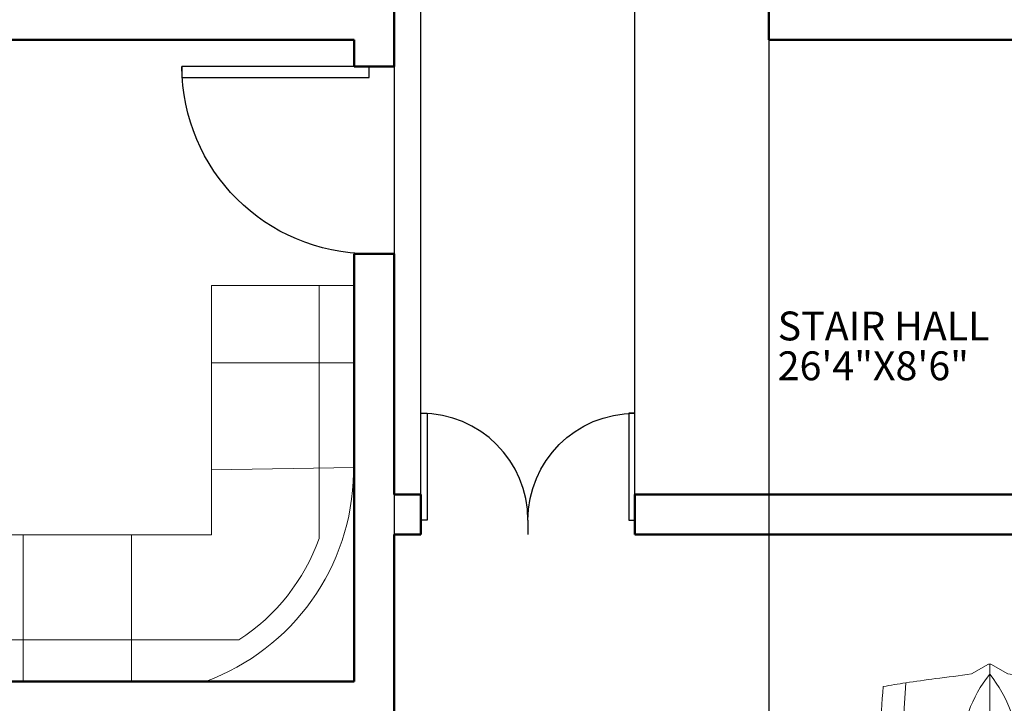
# Model space of a CAD drawing. Units: inches. Extents: x 5375 to 6084, y 16106 to 17259.
# Tile 8 of 32: x 5624 to 5844, y 16365 to 16518. Entities that reach past the tile are written whole.
import ezdxf

# ---------------------------------------------------------------- set-up
doc = ezdxf.new("R2010")
doc.units = ezdxf.units.IN
for name, color, linetype, lineweight in [('A-ANNO-DIMS', 2, 'Continuous', 18), ('A-AREA-IDEN', 5, 'Continuous', 18), ('C-PKNG-VEHI', 7, 'Continuous', 13), ('DOOR', 4, 'Continuous', 25), ('FURNITURE', 3, 'Continuous', 18), ('WALL', 6, 'Continuous', 50)]:
    doc.layers.add(name, color=color, linetype=linetype, lineweight=lineweight)
doc.styles.get("Standard").update_dxf_attribs({"font": 'arial.ttf'})
doc.dimstyles.get("Standard").update_dxf_attribs({"dimtxt": 0.18, "dimasz": 0.18, "dimexe": 0.18, "dimexo": 0.0625, "dimgap": 0.09, "dimtad": 0, "dimtih": 1, "dimtoh": 1, "dimdec": 4, "dimzin": 0, "dimdsep": 46, "dimtxsty": 'Standard', "dimcen": 0.09, "dimadec": 0, "dimazin": 0, "dimtfac": 1, "dimtdec": 4, "dimtofl": 0, "dimtmove": 0, "dimatfit": 3, "dimfxl": 1, "dimtolj": 1, "dimtzin": 0, "dimarcsym": 0})

# ---------------------------------------------------------------- blocks, each defined once
blk = doc.blocks.new('*U2')
for p, q in [((0, 0), (0, -100)), ((750, 0), (750, -100))]:
    blk.add_line(p, q)
blk.add_lwpolyline([(0, 0), (0, 750), (43.75, 750), (43.75, 0)], close=True)
blk.add_arc((0, 0), 750, 0, 90)
blk = doc.blocks.new('*U9')
for p, q in [((21.1, 37.41), (21.1, 36.83)), ((46.55, 38.89), (22.35, 38.89)), ((47.8, 37.39), (47.8, 37.41)), ((135.45, 37.07), (135.45, 37.41)), ((136.7, 38.89), (160.9, 38.89)), ((162.15, 37.41), (162.15, 36.77)), ((87.99, 31.87), (74.76, 35.92)), ((134.31, 35.6), (119.29, 31.78)), ((186.47, -33.5), (186.47, 33.5)), ((70.03, 31.54), (86.41, 29.35)), ((188.4, -32.76), (188.4, 32.76)), ((138.42, 29.35), (157.25, 29.35)), ((186.47, 29.35), (167.01, 29.35)), ((164.52, 26.39), (164.52, -26.39)), ((32.27, 11.63), (36.13, 17.17)), ((36.13, 17.17), (50.94, 17.17)), ((32.12, 9.51), (32.12, 11.15)), ((58.92, -10.77), (58.92, 10.77)), ((66.55, -10.53), (66.55, 10.53)), ((186.47, -10.53), (186.47, 10.53)), ((29.77, 9.51), (51.68, 9.51)), ((82.74, 8.5), (82.74, -8.5)), ((3.27, 6.13), (0.1, 0.41)), ((0, 0), (51.68, 0)), ((0.1, -0.41), (3.27, -6.13)), ((29.77, -9.51), (51.68, -9.51)), ((32.12, -9.51), (32.12, -11.15)), ((32.27, -11.63), (36.13, -17.17)), ((36.13, -17.17), (50.94, -17.17)), ((86.41, -29.35), (70.03, -31.54)), ((157.25, -29.35), (138.42, -29.35)), ((167.01, -29.35), (186.47, -29.35)), ((87.99, -31.87), (74.76, -35.92)), ((134.31, -35.6), (119.29, -31.78)), ((21.1, -37.41), (21.1, -36.83)), ((46.55, -38.89), (22.35, -38.89)), ((47.8, -37.39), (47.8, -37.41)), ((135.45, -37.07), (135.45, -37.41)), ((136.7, -38.89), (160.9, -38.89)), ((162.15, -37.41), (162.15, -36.77))]:
    blk.add_line(p, q)
for centre, major_axis, ratio, start_param, end_param in [((41.19, -490.86), (0, 528.23), 0.842304, 0.00281, 0.075598), ((22.35, 37.41), (0, -1.48), 0.842304, 3.141593, 4.712389), ((64.48, -10555.62), (0, 10593.03), 0.842304, -0.013397, 0.002797), ((46.55, 37.41), (0, 1.48), 0.842304, -1.570796, 0), ((136.7, 37.41), (0, -1.48), 0.842304, 3.141593, 4.712389), ((160.9, 37.41), (0, 1.48), 0.842304, -1.570796, 0), ((180.63, 35.84), (0, 2.22), 0.842304, -0.013017, 1.249894), ((64.48, -10556.36), (0, 10595.31), 0.842304, -0.013397, -0.013017), ((183.98, 32.76), (0, -5.25), 0.842304, 1.570796, 3.128196), ((266.03, -27.52), (0, 313.31), 0.842304, 1.367076, 1.39176), ((64.48, -10555.62), (0, -10591.55), 0.842304, 3.133765, 3.140441), ((183.98, 33.5), (0, -2.96), 0.842304, 1.570796, 3.128196), ((135.29, 5.39), (0, 81.77), 0.842304, 1.245306, 1.50788), ((95.79, -3666.35), (0, -3698.24), 0.842304, 3.134049, 3.144098), ((259.18, -27.52), (0, -305.3), 0.842304, 4.528606, 4.561838), ((37.47, -593.96), (0, -623.33), 0.842304, 3.096046, 3.200911), ((134.4, 5.39), (0, -89.78), 0.842304, 4.449482, 4.652344), ((149.6, 2.8), (0, -79.58), 0.842304, 4.372215, 4.640744), ((17.08, 0), (0, 147.02), 0.842304, 4.511394, 4.913384), ((35.91, 0), (0, 147.02), 0.842304, 4.511394, 4.913384), ((167.01, 26.39), (0, 2.96), 0.842304, 0, 1.570796), ((-204.49, 52.4), (0, -250.96), 0.842304, 1.385369, 1.434372), ((13.04, 17.01), (0, 27.42), 0.842304, 4.435146, 4.718221), ((14.2, 17.01), (0, 27.42), 0.842304, 4.435146, 4.718221), ((50.79, 13.34), (6.34, -0.36), 0.603834, -1.395552, 1.581315), ((32.75, 11.15), (0, 0.74), 0.842304, 0.879714, 1.570796), ((29.77, -46.66), (0, 56.17), 0.842304, 0, 0.590319), ((0.62, 0), (0, -0.74), 0.842304, 4.131459, 5.293319), ((29.77, 46.66), (0, 56.17), 0.842304, 2.551274, 3.141593), ((-204.49, -52.4), (0, 250.96), 0.842304, -1.434372, -1.385369), ((13.04, -17.01), (0, -27.42), 0.842304, 1.564964, 1.848039), ((14.2, -17.01), (0, -27.42), 0.842304, 1.564964, 1.848039), ((149.6, -2.8), (0, -79.58), 0.842304, -1.499151, -1.230623), ((32.75, -11.15), (0, -0.74), 0.842304, 4.712389, 5.403472), ((134.4, -5.39), (0, -89.78), 0.842304, -1.510751, -1.307889), ((135.29, -5.39), (0, -81.77), 0.842304, -1.50788, -1.245306), ((259.18, 27.52), (0, 305.3), 0.842304, 1.721348, 1.754579), ((167.01, -26.39), (0, -2.96), 0.842304, 4.712389, 6.283185), ((266.03, 27.52), (0, 313.31), 0.842304, 1.749832, 1.774517), ((37.47, 593.96), (0, -623.33), 0.842304, -0.059319, 0.045547), ((95.79, 3666.35), (0, -3698.24), 0.842304, -0.002505, 0.007544), ((183.98, -32.76), (0, -5.25), 0.842304, 0.013397, 1.570796), ((41.19, 490.86), (0, -528.23), 0.842304, -0.075598, -0.00281), ((64.48, 10555.62), (0, 10593.03), 0.842304, 3.138796, 3.15499), ((64.48, 10555.62), (0, -10591.55), 0.842304, 0.001152, 0.007828), ((183.98, -33.5), (0, 2.96), 0.842304, 3.15499, 4.712389), ((22.35, -37.41), (0, 1.48), 0.842304, 1.570796, 3.141593), ((46.55, -37.41), (0, -1.48), 0.842304, 0, 1.570796), ((136.7, -37.41), (0, -1.48), 0.842304, -1.570796, 0), ((160.9, -37.41), (0, 1.48), 0.842304, 3.141593, 4.712389), ((180.63, -35.84), (0, -2.22), 0.842304, -1.249894, 0.013017), ((64.48, 10556.36), (0, 10595.31), 0.842304, 3.15461, 3.15499)]:
    blk.add_ellipse(centre, major_axis=major_axis, ratio=ratio, start_param=start_param, end_param=end_param)
at = {"extrusion": (0, 0, -1)}
blk.add_ellipse((50.79, -13.34), major_axis=(6.34, 0.36), ratio=0.603834, start_param=-1.395552, end_param=1.581315, dxfattribs=at)
blk = doc.blocks.new('*D38')
at = {"layer": 'A-ANNO-DIMS', "color": 0, "lineweight": -2, "transparency": 16777216}
for p, q in [((5791.62, 16513.52), (5791.62, 16106.48)), ((5707.62, 16507.52), (5707.62, 16106.48)), ((5707.8, 16106.66), (5749.4, 16106.66)), ((5791.44, 16106.66), (5749.84, 16106.66))]:
    blk.add_line(p, q, dxfattribs=at)
at = {"layer": 'A-ANNO-DIMS', "color": 0, "transparency": 16777216}
for points in [[(5707.8, 16106.69), (5707.8, 16106.63), (5707.62, 16106.66)], [(5791.44, 16106.69), (5791.44, 16106.63), (5791.62, 16106.66)]]:
    blk.add_solid(points, dxfattribs=at)
at = {"layer": 'Defpoints', "color": 0, "transparency": 16777216}
for p in [(5791.62, 16513.58), (5707.62, 16507.58), (5791.62, 16106.66)]:
    blk.add_point(p, dxfattribs=at)
at = {"layer": 'A-ANNO-DIMS', "color": 0, "transparency": 16777216, "insert": (5749.62, 16106.66), "char_height": 0.18, "attachment_point": 5}
blk.add_mtext('\\A1;84', dxfattribs=at)
blk = doc.blocks.new('*D39')
at = {"layer": 'A-ANNO-DIMS', "color": 0, "lineweight": -2, "transparency": 16777216}
for p, q in [((5713.62, 16402.64), (5713.62, 17259.16)), ((5713.8, 17258.98), (5737.4, 17258.98)), ((5761.44, 17258.98), (5737.84, 17258.98)), ((5761.62, 16402.64), (5761.62, 17259.16))]:
    blk.add_line(p, q, dxfattribs=at)
at = {"layer": 'A-ANNO-DIMS', "color": 0, "transparency": 16777216}
for points in [[(5713.8, 17259.01), (5713.8, 17258.95), (5713.62, 17258.98)], [(5761.44, 17259.01), (5761.44, 17258.95), (5761.62, 17258.98)]]:
    blk.add_solid(points, dxfattribs=at)
at = {"layer": 'Defpoints', "color": 0, "transparency": 16777216}
for p in [(5761.62, 17258.98), (5713.62, 16402.58), (5761.62, 16402.58)]:
    blk.add_point(p, dxfattribs=at)
at = {"layer": 'A-ANNO-DIMS', "color": 0, "transparency": 16777216, "insert": (5737.62, 17258.98), "char_height": 0.18, "attachment_point": 5}
blk.add_mtext('\\A1;48', dxfattribs=at)

msp = doc.modelspace()

# ---------------------------------------------------------------- linework, layer by layer
at = {"layer": 'FURNITURE'}
for p, q in [((5666.6038, 16402.4975), (5666.6038, 16458.4398)), ((5666.6038, 16458.4398), (5698.6199, 16458.4398)), ((5690.7961, 16458.4398), (5690.7961, 16401.6723)), ((5666.6038, 16441.1015), (5698.6199, 16441.1015)), ((5666.6038, 16417.061), (5698.6199, 16417.5793)), ((5698.5058, 16416.3129), (5698.806, 16416.3129)), ((5520.2924, 16402.4975), (5666.6038, 16402.4975)), ((5624.3805, 16402.4975), (5624.3805, 16369.5793)), ((5648.6874, 16402.4975), (5648.6874, 16369.5793)), ((5520.2924, 16378.9228), (5672.8075, 16378.9228))]:
    msp.add_line(p, q, dxfattribs=at)
for radius, start, end in [(50.7384, 290.179605, 358.994547), (45.7384, 303.181366, 340.149946)]:
    msp.add_arc((5647.7752, 16417.2032), radius, start, end, dxfattribs=at)
at = {"layer": 'WALL'}
for p, q in [((5791.6199, 16690.5793), (5791.6199, 16513.5793)), ((5707.6199, 16642.5793), (5707.6199, 16507.5793)), ((5479.6199, 16513.5793), (5698.6199, 16513.5793)), ((5698.6199, 16513.5793), (5698.6199, 16507.5793)), ((5791.6199, 16513.5793), (6022.6199, 16513.5793)), ((5698.6199, 16507.5793), (5707.6199, 16507.5793)), ((5698.6199, 16465.5793), (5707.6199, 16465.5793)), ((5698.6199, 16465.5793), (5698.6199, 16369.5793)), ((5707.6199, 16465.5793), (5707.6199, 16411.5793)), ((5707.6199, 16411.5793), (5713.6199, 16411.5793)), ((5713.6199, 16411.5793), (5713.6199, 16402.5793)), ((5761.6199, 16411.5793), (5761.6199, 16402.5793)), ((5761.6199, 16411.5793), (6022.6199, 16411.5793)), ((5707.6199, 16402.5793), (5713.6199, 16402.5793)), ((5707.6199, 16402.5793), (5707.6199, 16360.5793)), ((5761.6199, 16402.5793), (6031.6199, 16402.5793)), ((5479.6199, 16369.5793), (5698.6199, 16369.5793))]:
    msp.add_line(p, q, dxfattribs=at)

# ---------------------------------------------------------------- block references
at = {"layer": 'C-PKNG-VEHI', "xscale": 0.6659567702331713, "yscale": 0.6659567702331713, "zscale": 0.6659567702331713, "rotation": 270}
msp.add_blockref('*U9', (5841.1969, 16373.5119), dxfattribs=at)
at = {"layer": 'DOOR', "xscale": -0.0559999999999998, "yscale": 0.0559999999999998, "zscale": 0.0559999999999998, "rotation": 90}
msp.add_blockref('*U2', (5702.0199, 16507.5793), dxfattribs=at)
at = {"layer": 'DOOR', "yscale": 0.0319999999999999, "zscale": 0.0319999999999999}
for p, xscale in [((5713.6199, 16405.7793), 0.0319999999999999), ((5761.6199, 16405.7793), -0.0319999999999999)]:
    msp.add_blockref('*U2', p, dxfattribs=dict(at, xscale=xscale))

# ---------------------------------------------------------------- texts
at = {"layer": 'A-AREA-IDEN'}
for s, p in [('STAIR HALL', (5793.6349, 16446.116)), ('26\'4"X8\'6"', (5793.6349, 16437.183))]:
    msp.add_text(s, height=6.47981, dxfattribs=at).set_placement(p)

# ---------------------------------------------------------------- dimensions: what is measured, and where the dimension line sits
at = {"layer": 'A-ANNO-DIMS'}
for base, p1, p2, picture, middle in [((5761.6199, 17258.9793), (5713.6199, 16402.5793), (5761.6199, 16402.5793), '*D39', (5737.6199, 17258.9793)), ((5791.6199, 16106.6631), (5707.6199, 16507.5793), (5791.6199, 16513.5793), '*D38', (5749.6199, 16106.6631))]:
    dim = msp.add_linear_dim(base=base, p1=p1, p2=p2, dimstyle='Standard', override={"dimdec": 0, "dimlfac": 1, "dimrnd": 0, "dimzin": 0, "dimdsep": 46, "dimlunit": 2}, dxfattribs=at)
    dim.commit()
    dim.dimension.update_dxf_attribs({"geometry": picture, "text_midpoint": middle})

doc.saveas('drawing.dxf')
